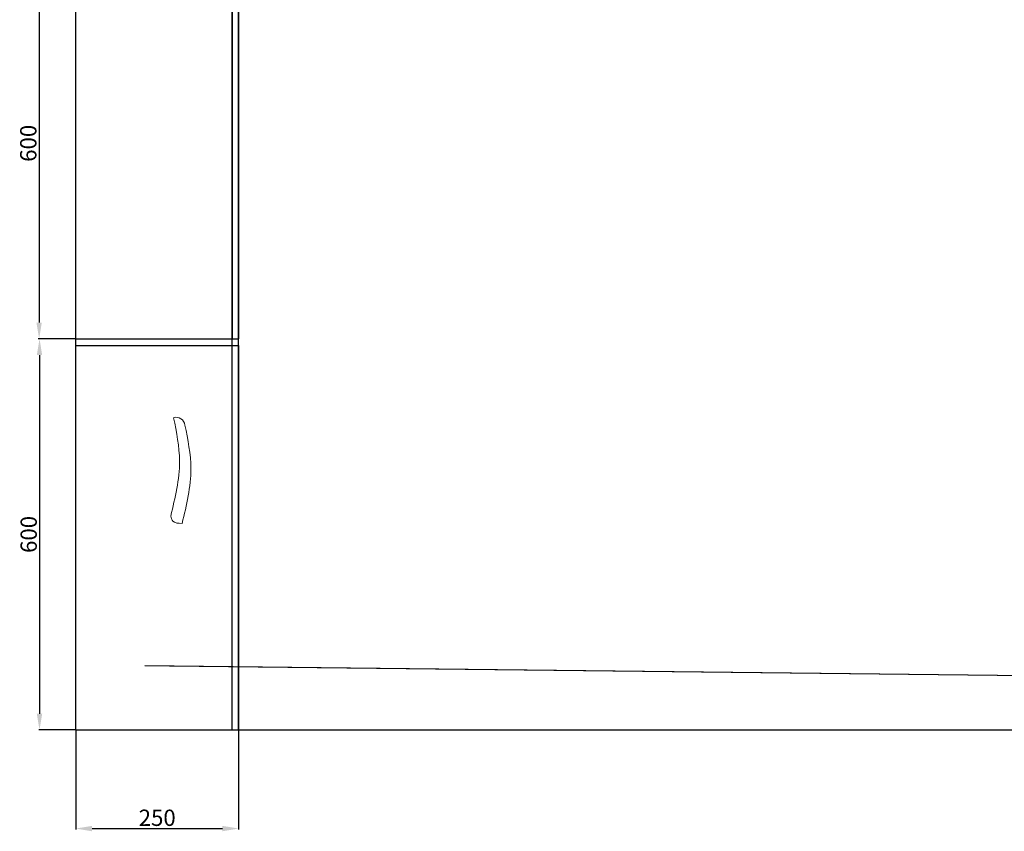
# Model space of a CAD drawing. Units: millimetres. Extents: x 11557 to 15272, y 8572 to 13242.
# Tile 1 of 4: x 11558 to 13069, y 9916 to 11161. Entities that reach past the tile are written whole.
import ezdxf

# ---------------------------------------------------------------- set-up
doc = ezdxf.new("R2010")
doc.units = ezdxf.units.MM
for name, color, linetype, lineweight in [('A-ANNO-DIMS', 2, 'Continuous', 18), ('A-FURN-HARD', 8, 'Continuous', 18), ('A-FURN-WALL', 7, 'Continuous', 30)]:
    doc.layers.add(name, color=color, linetype=linetype, lineweight=lineweight)
doc.styles.get("Standard").update_dxf_attribs({"font": 'arial.ttf'})
doc.dimstyles.new('ISO-25', dxfattribs={"dimtxt": 25, "dimasz": 25, "dimexe": 1.25, "dimexo": 0.625, "dimtad": 1, "dimdec": 1, "dimtxsty": 'Standard', "dimcen": 2.5, "dimadec": 0, "dimazin": 0, "dimtfac": 1, "dimtdec": 1, "dimtmove": 0, "dimatfit": 3, "dimfxl": 1, "dimarcsym": 0})

# ---------------------------------------------------------------- blocks, each defined once
blk = doc.blocks.new('*D7')
at = {"layer": 'A-ANNO-DIMS', "color": 0, "lineweight": -2, "transparency": 16777216}
for p, q in [((11643.8, 10671.7), (11587.5, 10671.7)), ((11588.8, 10646.7), (11588.8, 10096.7)), ((11643.8, 10071.7), (11587.5, 10071.7))]:
    blk.add_line(p, q, dxfattribs=at)
at = {"layer": 'A-ANNO-DIMS', "color": 0, "transparency": 16777216}
for points in [[(11584.6, 10646.7), (11592.9, 10646.7), (11588.8, 10671.7)], [(11584.6, 10096.7), (11592.9, 10096.7), (11588.8, 10071.7)]]:
    blk.add_solid(points, dxfattribs=at)
at = {"layer": 'Defpoints', "color": 0, "transparency": 16777216}
for p in [(11644.4, 10671.7, 720), (11588.8, 10071.7), (11644.4, 10071.7, 720)]:
    blk.add_point(p, dxfattribs=at)
at = {"layer": 'A-ANNO-DIMS', "color": 0, "transparency": 16777216, "insert": (11575.4, 10371.7), "char_height": 25, "attachment_point": 5, "rotation": 90}
blk.add_mtext('600', dxfattribs=at)
blk = doc.blocks.new('*D8')
at = {"layer": 'A-ANNO-DIMS', "color": 0, "lineweight": -2, "transparency": 16777216}
for p, q in [((11643.1, 11271.7), (11586.9, 11271.7)), ((11588.2, 11246.7), (11588.2, 10696.7)), ((11643.1, 10671.7), (11586.9, 10671.7))]:
    blk.add_line(p, q, dxfattribs=at)
at = {"layer": 'A-ANNO-DIMS', "color": 0, "transparency": 16777216}
for points in [[(11584, 11246.7), (11592.3, 11246.7), (11588.2, 11271.7)], [(11584, 10696.7), (11592.3, 10696.7), (11588.2, 10671.7)]]:
    blk.add_solid(points, dxfattribs=at)
at = {"layer": 'Defpoints', "color": 0, "transparency": 16777216}
for p in [(11643.8, 11271.7, 720), (11588.2, 10671.7), (11643.8, 10671.7, 720)]:
    blk.add_point(p, dxfattribs=at)
at = {"layer": 'A-ANNO-DIMS', "color": 0, "transparency": 16777216, "insert": (11574.8, 10971.7), "char_height": 25, "attachment_point": 5, "rotation": 90}
blk.add_mtext('600', dxfattribs=at)
blk = doc.blocks.new('*D34')
at = {"layer": 'A-ANNO-DIMS', "color": 0, "lineweight": -2, "transparency": 16777216}
for p, q in [((11644.4, 10071), (11644.4, 9919.2)), ((11894.4, 10071), (11894.4, 9919.2)), ((11669.4, 9920.5), (11869.4, 9920.5))]:
    blk.add_line(p, q, dxfattribs=at)
at = {"layer": 'A-ANNO-DIMS', "color": 0, "transparency": 16777216}
for points in [[(11669.4, 9924.6), (11669.4, 9916.3), (11644.4, 9920.5)], [(11869.4, 9924.6), (11869.4, 9916.3), (11894.4, 9920.5)]]:
    blk.add_solid(points, dxfattribs=at)
at = {"layer": 'Defpoints', "color": 0, "transparency": 16777216}
for p in [(11644.4, 10071.7), (11894.4, 10071.7), (11894.4, 9920.5)]:
    blk.add_point(p, dxfattribs=at)
at = {"layer": 'A-ANNO-DIMS', "color": 0, "transparency": 16777216, "insert": (11769.4, 9933.8), "char_height": 25, "attachment_point": 5}
blk.add_mtext('250', dxfattribs=at)
blk = doc.blocks.new('*D36')
at = {"layer": 'A-ANNO-DIMS', "color": 0, "lineweight": -2, "transparency": 16777216}
for p, q in [((12944.4, 13071.7), (13209.3, 13071.7)), ((13208.1, 10096.7), (13208.1, 13046.7)), ((11895, 10071.7), (13209.3, 10071.7))]:
    blk.add_line(p, q, dxfattribs=at)
at = {"layer": 'A-ANNO-DIMS', "color": 0, "transparency": 16777216}
for points in [[(13203.9, 13046.7), (13212.2, 13046.7), (13208.1, 13071.7)], [(13203.9, 10096.7), (13212.2, 10096.7), (13208.1, 10071.7)]]:
    blk.add_solid(points, dxfattribs=at)
at = {"layer": 'Defpoints', "color": 0, "transparency": 16777216}
for p in [(12943.8, 13071.7), (13208.1, 13071.7), (11894.4, 10071.7)]:
    blk.add_point(p, dxfattribs=at)
at = {"layer": 'A-ANNO-DIMS', "color": 0, "transparency": 16777216, "insert": (13194.7, 11571.7), "char_height": 25, "attachment_point": 5, "rotation": 90}
blk.add_mtext('3000', dxfattribs=at)
blk = doc.blocks.new('*D52')
at = {"layer": 'A-ANNO-DIMS', "color": 0, "lineweight": -2, "transparency": 16777216}
for p, q in [((11750.2, 10170.7), (13738.5, 10148.2)), ((14995.9, 10133.9), (13763.5, 10147.9))]:
    blk.add_line(p, q, dxfattribs=at)
at = {"layer": 'A-ANNO-DIMS', "color": 0, "transparency": 16777216}
blk.add_solid([(13763.5, 10152), (13763.4, 10143.7), (13738.5, 10148.2)], dxfattribs=at)
at = {"layer": 'Defpoints', "color": 0, "transparency": 16777216}
for p in [(11750.2, 10170.7), (13738.5, 10148.2)]:
    blk.add_point(p, dxfattribs=at)
at = {"layer": 'A-ANNO-DIMS', "color": 0, "transparency": 16777216, "insert": (14931.6, 10148), "char_height": 25, "attachment_point": 5, "rotation": 359.3508}
blk.add_mtext('R1988.4', dxfattribs=at)
blk = doc.blocks.new('*D53')
at = {"layer": 'A-ANNO-DIMS', "color": 0, "lineweight": -2, "transparency": 16777216}
for p, q in [((11788.3, 10170.3), (13738.8, 10148.2)), ((14973.5, 10134.2), (13763.8, 10147.9))]:
    blk.add_line(p, q, dxfattribs=at)
at = {"layer": 'A-ANNO-DIMS', "color": 0, "transparency": 16777216}
blk.add_solid([(13763.8, 10152), (13763.7, 10143.7), (13738.8, 10148.2)], dxfattribs=at)
at = {"layer": 'Defpoints', "color": 0, "transparency": 16777216}
for p in [(11788.3, 10170.3), (13738.8, 10148.2)]:
    blk.add_point(p, dxfattribs=at)
at = {"layer": 'A-ANNO-DIMS', "color": 0, "transparency": 16777216, "insert": (14909.2, 10148.3), "char_height": 25, "attachment_point": 5, "rotation": 359.3508}
blk.add_mtext('R1950.6', dxfattribs=at)

msp = doc.modelspace()

# ---------------------------------------------------------------- linework, layer by layer
at = {"layer": 'A-FURN-HARD'}
msp.add_arc((11798.368, 10537.606, -110), 13.754, 7.963069, 106.22766, dxfattribs=at)
for points, knots in [([(11790.064, 10399.931, -110), (11796.916, 10427.938, -110), (11809.187, 10478.1, -110), (11799.016, 10528.536, -110), (11794.524, 10550.812, -110)], [0, 0, 0, 0, 85.19241077, 152.5838034, 152.5838034, 152.5838034, 152.5838034]), ([(11807.529, 10388.631, -110), (11814.38, 10416.638, -110), (11826.651, 10466.8, -110), (11816.481, 10517.236, -110), (11811.989, 10539.512, -110)], [0, 0, 0, 0, 85.19241077, 152.5838034, 152.5838034, 152.5838034, 152.5838034]), ([(11790.064, 10399.931, -110), (11790.806, 10397.027, -110), (11792.869, 10388.943, -110), (11801.804, 10388.753, -110), (11807.529, 10388.631, -110)], [0, 0, 0, 0, 8.29929483, 23.09865067, 23.09865067, 23.09865067, 23.09865067])]:
    msp.add_open_spline(points, degree=3, knots=knots, dxfattribs=at)
at = {"layer": 'A-FURN-WALL'}
for p, q in [((11644.396, 10671.656, 250), (11644.396, 11271.656, 250)), ((11884.396, 11271.656, 250), (11884.396, 10671.656, 250)), ((11884.396, 10671.656, 250), (11884.396, 11271.656, 250)), ((11894.396, 11271.656, 250), (11894.396, 10671.656, 250)), ((11894.396, 10671.656, 250), (11894.396, 11271.656, 250)), ((11894.396, 10671.656, -470), (11894.396, 11271.656, -470)), ((11894.396, 10971.656, 250), (11894.396, 10971.656, -470)), ((11644.396, 10071.656, 250), (11644.396, 10671.656, 250)), ((11644.396, 10671.656, 250), (11894.396, 10671.656, 250)), ((11884.396, 10071.656, 250), (11884.396, 10671.656, 250)), ((11894.396, 10071.656, 250), (11894.396, 10671.656, 250)), ((11894.396, 10671.656, 250), (11894.396, 10671.656, -470)), ((11894.396, 10661.656, -470), (11894.396, 10671.656, -470)), ((11644.396, 10661.656, 250), (11894.396, 10661.656, 250)), ((11644.396, 10661.656, -360), (11644.396, 10661.656, -470)), ((11644.396, 10661.656, -470), (11894.396, 10661.656, -470)), ((11644.396, 10661.656, -460), (11894.396, 10661.656, -460)), ((11894.396, 10661.656, 250), (11894.396, 10661.656, -470)), ((11894.396, 10661.656, -110), (11894.396, 10071.656, -110)), ((11894.396, 10071.656, 250), (11644.396, 10071.656, 250)), ((11644.396, 10071.656, 250), (11644.396, 10071.656, -110)), ((11894.396, 10071.656, 239.77), (11644.396, 10071.656, 239.77)), ((11884.396, 10071.656, -110), (11644.396, 10071.656, -110)), ((11884.396, 10071.656, -110), (11884.396, 10071.656, 250)), ((11894.396, 10071.656, -110), (11884.396, 10071.656, -110)), ((11894.396, 10071.656, -110), (11894.396, 10071.656, 250))]:
    msp.add_line(p, q, dxfattribs=at)

# ---------------------------------------------------------------- dimensions: what is measured, and where the dimension line sits
at = {"layer": 'A-ANNO-DIMS'}
dim = msp.add_linear_dim(base=(13208.076, 13071.656), p1=(11894.396, 10071.656), p2=(12943.771, 13071.656), angle=90, dimstyle='ISO-25', override={"dimdec": 0, "dimlfac": 1, "dimrnd": 0, "dimzin": 0, "dimdsep": 46, "dimlunit": 2}, dxfattribs=at)
dim.commit()
dim.dimension.update_dxf_attribs({"geometry": '*D36', "text_midpoint": (13194.678, 11571.656)})
for base, p1, p2, picture, middle in [((11588.151, 10671.656, 250), (11643.771, 11271.656, 970), (11643.771, 10671.656, 970), '*D8', (11588.151, 10971.656, 250)), ((11588.776, 10071.656, 250), (11644.396, 10671.656, 970), (11644.396, 10071.656, 970), '*D7', (11588.776, 10371.656, 250))]:
    dim = msp.add_linear_dim(base=base, p1=p1, p2=p2, angle=90, dimstyle='ISO-25', override={"dimclrd": 0, "dimclre": 0, "dimclrt": 0}, dxfattribs=at)
    dim.commit()
    dim.dimension.update_dxf_attribs({"geometry": picture, "text_midpoint": middle, "dimtype": 160})
for center, mpoint, picture, middle in [((11750.209, 10170.692), (13738.481, 10148.164), '*D52', (14931.444, 10134.647)), ((11788.258, 10170.261), (13738.772, 10148.161), '*D53', (14909.08, 10134.901))]:
    dim = msp.add_radius_dim(center=center, mpoint=mpoint, dimstyle='ISO-25', override={"dimdec": 1, "dimlfac": 1, "dimrnd": 0, "dimzin": 0, "dimdsep": 46, "dimlunit": 2}, dxfattribs=at)
    dim.commit()
    dim.dimension.update_dxf_attribs({"geometry": picture, "text_midpoint": middle, "dimtype": 164})
dim = msp.add_linear_dim(base=(11894.396, 9920.456), p1=(11644.396, 10071.656), p2=(11894.396, 10071.656), dimstyle='ISO-25', override={"dimdec": 0, "dimlfac": 1, "dimrnd": 0, "dimzin": 0, "dimdsep": 46, "dimlunit": 2}, dxfattribs=at)
dim.commit()
dim.dimension.update_dxf_attribs({"geometry": '*D34', "text_midpoint": (11769.396, 9933.846)})

doc.saveas('drawing.dxf')
